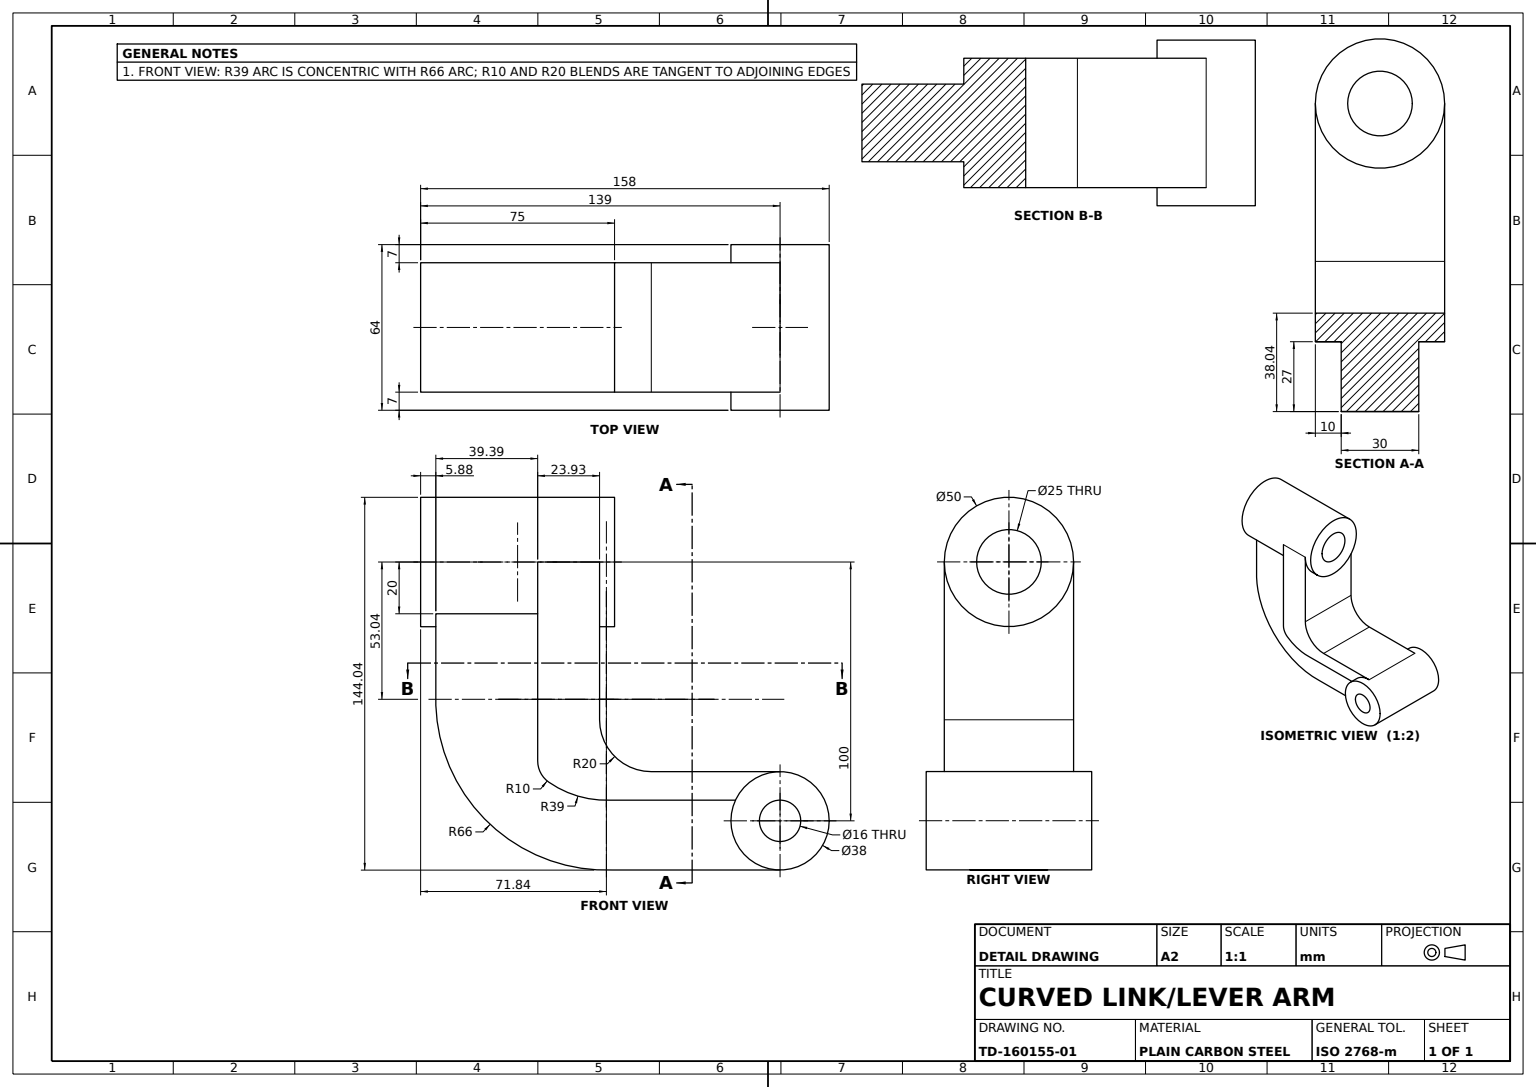
SolidWorks part; units mm, degrees
material "Plain Carbon Steel"
ref_plane "Front Plane" through (0, 0, 0) normal (0, 0, 1) x (1, 0, 0)
ref_plane "Top Plane" through (0, 0, 0) normal (0, 1, 0) x (1, 0, 0)
ref_plane "Right Plane" through (0, 0, 0) normal (1, 0, 0) x (0, 0, -1)
sketch "Hub 1 Profile" plane through (0, 0, 0) normal (1, 0, 0) x (0, 0, -1)
  circle A0 centre (0, 0) radius 25
  dimension "D1" = 50
extrude "Hub 1 Boss 75mm" add sketch "Hub 1 Profile" along normal mid plane 75
sketch "Hub 2 Profile" plane through (0, 0, 0) normal (0, 0, 1) x (1, 0, 0)
  line L0 (37.5, 0) -> (37.5, -100)
  line L1 (37.5, -25) -> (37.5, 25) construction
  line L2 (37.5, -100) -> (101.5, -100)
  circle A0 centre (101.5, -100) radius 19
  dimension "D1" = 38
  dimension "D2" = 64
  dimension "D3" = 100
extrude "Hub 2 Boss 64mm" add sketch "Hub 2 Profile" along normal mid plane 64 separate body
sketch "Curved Arm Profile" plane through (0, 0, 0) normal (0, 0, 1) x (1, 0, 0)
  line L0 (101.5, -119) -> (36.7078, -119)
  line L2 (-37.5, -25) -> (37.5, -25) construction
  line L3 (-31.6183, -25) -> (-31.6183, -55.4112)
  line L4 (35.7388, -92.0174) -> (84.2582, -92.0174)
  line L6 (-31.6183, -25) -> (-31.6183, -18.704)
  line L9 (84.2582, -92.0174) -> (91.481, -92.0174)
  line L10 (101.5, -119) -> (101.5, -92.0174)
  line L11 (101.5, -92.0174) -> (91.481, -92.0174)
  line L12 (-31.6183, -18.704) -> (7.7695, -18.704)
  line L13 (7.7695, -18.704) -> (7.7695, -76.8426)
  circle A0 centre (101.5, -100) radius 19 construction
  arc A2 (36.7078, -119) -> (-31.6183, -55.4112) centre (34.3392, -53.0425) cw
  arc A3 (35.7388, -92.0174) -> (12.0558, -85.0496) centre (34.3392, -53.0425) cw
  arc A4 (101.5, -119) -> (84.2582, -92.0174) centre (101.5, -100) cw
  arc A5 (7.7695, -76.8426) -> (12.0558, -85.0496) centre (17.7695, -76.8426) ccw
  arc A6 (35.7388, -92.0174) -> (-4.6357, -54.4422) centre (34.3392, -53.0425) cw construction
  dimension "D3" = 27
  dimension "D1" = 10
  dimension "D4" = 66
  dimension "D5" = 19
  dimension "D6" = 39.3878
  dimension "D2" = 119
  dimension "D7" = 43.6741
  dimension "D8" = 67.3572
  dimension "D9" = 115.8766
  dimension "D10" = 123.0993
  dimension "D11" = 100.296
extrude "Curved Arm Web" add sketch "Curved Arm Profile" along normal mid plane 30
sketch "Arm Flange Profile" plane through (0, 0, 0) normal (0, 0, 1) x (1, 0, 0)
  line L1 (31.7044, -20) -> (31.7044, -61)
  line L2 (51.7044, -81) -> (101.5, -81)
  line L3 (7.7695, -20) -> (7.7695, -76.8426)
  line L4 (35.7388, -92.0174) -> (84.2582, -92.0174)
  line L5 (7.7695, -20) -> (7.7695, 0)
  line L6 (7.7695, 0) -> (31.7044, 0)
  line L7 (31.7044, 0) -> (31.7044, -20)
  circle A0 centre (101.5, -100) radius 19 construction
  arc A1 (31.7044, -61) -> (51.7044, -81) centre (51.7044, -61) ccw
  arc A2 (7.7695, -76.8426) -> (12.0558, -85.0496) centre (17.7695, -76.8426) ccw
  arc A3 (12.0558, -85.0496) -> (35.7388, -92.0174) centre (34.3392, -53.0425) ccw
  arc A4 (84.2582, -92.0174) -> (101.5, -81) centre (101.5, -100) cw
  dimension "D1" = 20
  dimension "D2" = 10
  dimension "D3" = 39
  dimension "D4" = 23.935
  dimension "D5" = 20
  dimension "D6" = 53.0425
extrude "Arm Flange" add sketch "Arm Flange Profile" along normal mid plane 50
sketch "Hub 1 Bore Profile" plane through (37.5, 0, 0) normal (1, 0, 0) x (0, 0, -1)
  circle A0 centre (0, 0) radius 12.5
  dimension "D1" = 25
extrude "Hub 1 Bore" cut sketch "Hub 1 Bore Profile" against normal blind 88
sketch "Hub 2 Bore Profile" plane through (0, 0, -32) normal (0, 0, -1) x (-1, 0, 0)
  circle A0 centre (-101.5, -100) radius 8
  dimension "D1" = 16
extrude "Hub 2 Bore" cut sketch "Hub 2 Bore Profile" against normal blind 88
